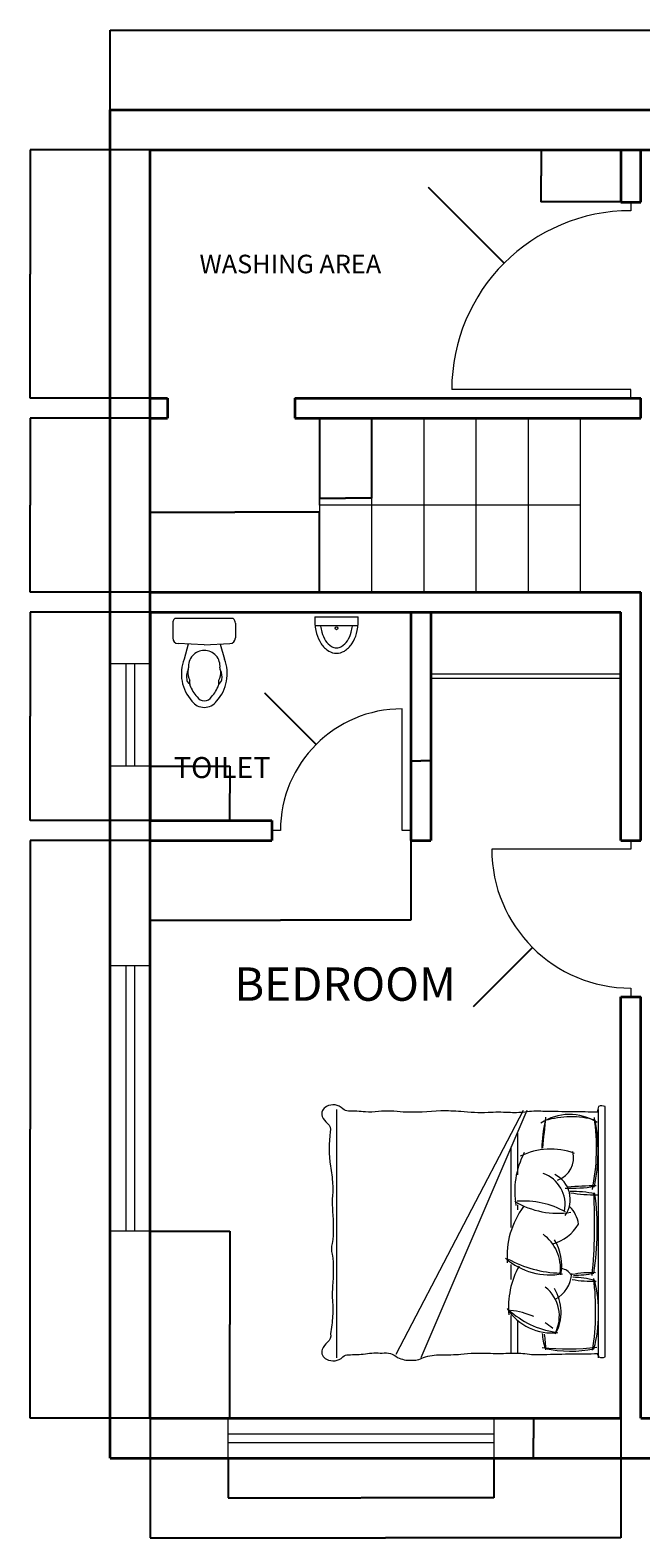
# Model space of a CAD drawing. Units: millimetres. Extents: x 2511 to 24632, y 2213 to 12972.
# Tile 1 of 5: x 2511 to 6023, y 2213 to 10891. Entities that reach past the tile are written whole.
import ezdxf

# ---------------------------------------------------------------- set-up
doc = ezdxf.new("R2010")
doc.units = ezdxf.units.MM
for name, color, linetype, lineweight in [('A-ANNO-DIMS', 2, 'Continuous', 18), ('A-AREA-IDEN', 7, 'Continuous', 20), ('A-FLOR-CASE', 7, 'Continuous', 18), ('A-FLOR-FIXT', 5, 'Continuous', 18), ('A-FLOR-STRS', 7, 'Continuous', 18), ('A-WALL', 7, 'Continuous', 35), ('doors', 50, 'Continuous', 18), ('windows', 70, 'Continuous', 18)]:
    doc.layers.add(name, color=color, linetype=linetype, lineweight=lineweight)
doc.layers.add('A-FURN', color=11, linetype='Continuous', lineweight=18, true_color=0xf27172)
doc.styles.get("Standard").update_dxf_attribs({"font": 'arial.ttf'})
doc.dimstyles.get("Standard").update_dxf_attribs({"dimtxt": 0.18, "dimasz": 0.18, "dimexe": 0.18, "dimexo": 0.0625, "dimgap": 0.09, "dimtad": 0, "dimtih": 1, "dimtoh": 1, "dimdec": 4, "dimzin": 0, "dimdsep": 46, "dimtxsty": 'Standard', "dimcen": 0.09, "dimadec": 0, "dimazin": 0, "dimtfac": 1, "dimtdec": 4, "dimtofl": 0, "dimtmove": 0, "dimatfit": 3, "dimfxl": 1, "dimtolj": 1, "dimtzin": 0, "dimarcsym": 0})

# ---------------------------------------------------------------- blocks, each defined once
blk = doc.blocks.new('WINDOW-1528-PLAN')
for p, q in [((0, 140), (1528, 140)), ((0, 90), (1528, 90))]:
    blk.add_line(p, q)
blk.add_lwpolyline([(0, 230), (1528, 230), (1528, 0), (0, 0)], close=True)
blk = doc.blocks.new('WINDOW-592-PLAN')
for p, q in [((0, 140), (591.5, 140)), ((0, 90), (591.5, 90))]:
    blk.add_line(p, q)
blk.add_lwpolyline([(0, 230), (591.5, 230), (591.5, 0), (0, 0)], close=True)
blk = doc.blocks.new('*D19')
at = {"layer": 'A-ANNO-DIMS', "color": 0, "lineweight": -2, "transparency": 16777216}
for p, q in [((3649.2, 2671.8), (3649.2, 2442.5)), ((5177.2, 2671.8), (5177.2, 2442.5)), ((3649.4, 2442.7), (4412, 2442.7)), ((5177, 2442.7), (4414.5, 2442.7))]:
    blk.add_line(p, q, dxfattribs=at)
at = {"layer": 'A-ANNO-DIMS', "color": 0, "transparency": 16777216}
for points in [[(3649.4, 2442.7), (3649.4, 2442.6), (3649.2, 2442.7)], [(5177, 2442.7), (5177, 2442.6), (5177.2, 2442.7)]]:
    blk.add_solid(points, dxfattribs=at)
at = {"layer": 'Defpoints', "color": 0, "transparency": 16777216}
for p in [(3649.2, 2671.9), (5177.2, 2671.9), (5177.2, 2442.7)]:
    blk.add_point(p, dxfattribs=at)
at = {"layer": 'A-ANNO-DIMS', "color": 0, "transparency": 16777216, "insert": (4413.2, 2442.7), "char_height": 0.18, "attachment_point": 5}
blk.add_mtext('\\A1;WINDOW 1528 TYP.', dxfattribs=at)
blk = doc.blocks.new('*D20')
at = {"layer": 'A-ANNO-DIMS', "color": 0, "lineweight": -2, "transparency": 16777216}
for p, q in [((5177.3, 2901.9), (5406.6, 2901.9)), ((5406.4, 2901.7), (5406.4, 2787)), ((5406.4, 2672), (5406.4, 2786.7)), ((5177.3, 2671.9), (5406.6, 2671.9))]:
    blk.add_line(p, q, dxfattribs=at)
at = {"layer": 'A-ANNO-DIMS', "color": 0, "transparency": 16777216}
for points in [[(5406.4, 2901.7), (5406.4, 2901.7), (5406.4, 2901.9)], [(5406.4, 2672), (5406.4, 2672), (5406.4, 2671.9)]]:
    blk.add_solid(points, dxfattribs=at)
at = {"layer": 'Defpoints', "color": 0, "transparency": 16777216}
for p in [(5177.2, 2901.9), (5406.4, 2901.9), (5177.2, 2671.9)]:
    blk.add_point(p, dxfattribs=at)
at = {"layer": 'A-ANNO-DIMS', "color": 0, "transparency": 16777216, "insert": (5406.4, 2786.9), "char_height": 0.18, "attachment_point": 5}
blk.add_mtext('\\A1;230 TYP.', dxfattribs=at)
blk = doc.blocks.new('*D35')
at = {"layer": 'A-ANNO-DIMS', "color": 0, "lineweight": -2, "transparency": 16777216}
for p, q in [((2970.2, 10431.9), (2970.2, 10891)), ((2970.4, 10890.9), (7557.9, 10890.9)), ((12146, 10890.9), (7558.6, 10890.9)), ((12146.2, 7356.9), (12146.2, 10891))]:
    blk.add_line(p, q, dxfattribs=at)
at = {"layer": 'A-ANNO-DIMS', "color": 0, "transparency": 16777216}
for points in [[(2970.4, 10890.9), (2970.4, 10890.8), (2970.2, 10890.9)], [(12146, 10890.9), (12146, 10890.8), (12146.2, 10890.9)]]:
    blk.add_solid(points, dxfattribs=at)
at = {"layer": 'Defpoints', "color": 0, "transparency": 16777216}
for p in [(12146.2, 10890.9), (2970.2, 10431.9), (12146.2, 7356.9)]:
    blk.add_point(p, dxfattribs=at)
at = {"layer": 'A-ANNO-DIMS', "color": 0, "transparency": 16777216, "insert": (7558.2, 10890.9), "char_height": 0.18, "attachment_point": 5}
blk.add_mtext('\\A1;9176', dxfattribs=at)
blk = doc.blocks.new('*D37')
at = {"layer": 'A-ANNO-DIMS', "color": 0, "lineweight": -2, "transparency": 16777216}
for p, q in [((3200.2, 2901.8), (3200.2, 2212.7)), ((5908.2, 2901.8), (5908.2, 2212.7)), ((3200.4, 2212.9), (4553.9, 2212.9)), ((5908, 2212.9), (4554.6, 2212.9))]:
    blk.add_line(p, q, dxfattribs=at)
at = {"layer": 'A-ANNO-DIMS', "color": 0, "transparency": 16777216}
for points in [[(3200.4, 2212.9), (3200.4, 2212.8), (3200.2, 2212.9)], [(5908, 2212.9), (5908, 2212.8), (5908.2, 2212.9)]]:
    blk.add_solid(points, dxfattribs=at)
at = {"layer": 'Defpoints', "color": 0, "transparency": 16777216}
for p in [(3200.2, 2901.9), (5908.2, 2901.9), (5908.2, 2212.9)]:
    blk.add_point(p, dxfattribs=at)
at = {"layer": 'A-ANNO-DIMS', "color": 0, "transparency": 16777216, "insert": (4554.2, 2212.9), "char_height": 0.18, "attachment_point": 5}
blk.add_mtext('\\A1;2708', dxfattribs=at)
blk = doc.blocks.new('*D40')
at = {"layer": 'A-ANNO-DIMS', "color": 0, "lineweight": -2, "transparency": 16777216}
for p, q in [((3200.2, 6226.9), (2511, 6226.9)), ((2511.2, 6226.7), (2511.2, 4564.5)), ((2511.2, 2902), (2511.2, 4564.2)), ((3200.2, 2901.9), (2511, 2901.9))]:
    blk.add_line(p, q, dxfattribs=at)
at = {"layer": 'A-ANNO-DIMS', "color": 0, "transparency": 16777216}
for points in [[(2511.2, 6226.7), (2511.2, 6226.7), (2511.2, 6226.9)], [(2511.2, 2902), (2511.2, 2902), (2511.2, 2901.9)]]:
    blk.add_solid(points, dxfattribs=at)
at = {"layer": 'Defpoints', "color": 0, "transparency": 16777216}
for p in [(2511.2, 6226.9), (3200.2, 6226.9), (3200.2, 2901.9)]:
    blk.add_point(p, dxfattribs=at)
at = {"layer": 'A-ANNO-DIMS', "color": 0, "transparency": 16777216, "insert": (2511.2, 4564.4), "char_height": 0.18, "attachment_point": 5}
blk.add_mtext('\\A1;3325', dxfattribs=at)
blk = doc.blocks.new('*D41')
at = {"layer": 'A-ANNO-DIMS', "color": 0, "lineweight": -2, "transparency": 16777216}
for p, q in [((3200.2, 7541.9), (2511, 7541.9)), ((2511.2, 7541.7), (2511.2, 6942)), ((2511.2, 6342), (2511.2, 6941.7)), ((3200.2, 6341.9), (2511, 6341.9))]:
    blk.add_line(p, q, dxfattribs=at)
at = {"layer": 'A-ANNO-DIMS', "color": 0, "transparency": 16777216}
for points in [[(2511.2, 7541.7), (2511.2, 7541.7), (2511.2, 7541.9)], [(2511.2, 6342), (2511.2, 6342), (2511.2, 6341.9)]]:
    blk.add_solid(points, dxfattribs=at)
at = {"layer": 'Defpoints', "color": 0, "transparency": 16777216}
for p in [(2511.2, 7541.9), (3200.2, 7541.9), (3200.2, 6341.9)]:
    blk.add_point(p, dxfattribs=at)
at = {"layer": 'A-ANNO-DIMS', "color": 0, "transparency": 16777216, "insert": (2511.2, 6941.9), "char_height": 0.18, "attachment_point": 5}
blk.add_mtext('\\A1;1200', dxfattribs=at)
blk = doc.blocks.new('*D42')
at = {"layer": 'A-ANNO-DIMS', "color": 0, "lineweight": -2, "transparency": 16777216}
for p, q in [((3200.2, 8656.9), (2511, 8656.9)), ((2511.2, 8656.7), (2511.2, 8157)), ((2511.2, 7657), (2511.2, 8156.7)), ((3200.2, 7656.9), (2511, 7656.9))]:
    blk.add_line(p, q, dxfattribs=at)
at = {"layer": 'A-ANNO-DIMS', "color": 0, "transparency": 16777216}
for points in [[(2511.2, 8656.7), (2511.2, 8656.7), (2511.2, 8656.9)], [(2511.2, 7657), (2511.2, 7657), (2511.2, 7656.9)]]:
    blk.add_solid(points, dxfattribs=at)
at = {"layer": 'Defpoints', "color": 0, "transparency": 16777216}
for p in [(2511.2, 8656.9), (3200.2, 8656.9), (3200.2, 7656.9)]:
    blk.add_point(p, dxfattribs=at)
at = {"layer": 'A-ANNO-DIMS', "color": 0, "transparency": 16777216, "insert": (2511.2, 8156.9), "char_height": 0.18, "attachment_point": 5}
blk.add_mtext('\\A1;1000', dxfattribs=at)
blk = doc.blocks.new('*D43')
at = {"layer": 'A-ANNO-DIMS', "color": 0, "lineweight": -2, "transparency": 16777216}
for p, q in [((3200.2, 10201.9), (2511, 10201.9)), ((2511.2, 10201.7), (2511.2, 9487)), ((2511.2, 8772), (2511.2, 9486.7)), ((3200.2, 8771.9), (2511, 8771.9))]:
    blk.add_line(p, q, dxfattribs=at)
at = {"layer": 'A-ANNO-DIMS', "color": 0, "transparency": 16777216}
for points in [[(2511.2, 10201.7), (2511.2, 10201.7), (2511.2, 10201.9)], [(2511.2, 8772), (2511.2, 8772), (2511.2, 8771.9)]]:
    blk.add_solid(points, dxfattribs=at)
at = {"layer": 'Defpoints', "color": 0, "transparency": 16777216}
for p in [(2511.2, 10201.9), (3200.2, 10201.9), (3200.2, 8771.9)]:
    blk.add_point(p, dxfattribs=at)
at = {"layer": 'A-ANNO-DIMS', "color": 0, "transparency": 16777216, "insert": (2511.2, 9486.9), "char_height": 0.18, "attachment_point": 5}
blk.add_mtext('\\A1;1430', dxfattribs=at)
blk = doc.blocks.new('*D44')
at = {"layer": 'A-ANNO-DIMS', "color": 0, "lineweight": -2, "transparency": 16777216}
for p, q in [((3200.3, 3978.2), (3659.4, 3978.2)), ((3659.2, 3978), (3659.2, 3440.2)), ((3659.2, 2902), (3659.2, 3439.9)), ((3200.3, 2901.9), (3659.4, 2901.9))]:
    blk.add_line(p, q, dxfattribs=at)
at = {"layer": 'A-ANNO-DIMS', "color": 0, "transparency": 16777216}
for points in [[(3659.2, 3978), (3659.2, 3978), (3659.2, 3978.2)], [(3659.2, 2902), (3659.2, 2902), (3659.2, 2901.9)]]:
    blk.add_solid(points, dxfattribs=at)
at = {"layer": 'Defpoints', "color": 0, "transparency": 16777216}
for p in [(3200.2, 3978.2), (3200.2, 2901.9), (3659.2, 2901.9)]:
    blk.add_point(p, dxfattribs=at)
at = {"layer": 'A-ANNO-DIMS', "color": 0, "transparency": 16777216, "insert": (3659.2, 3440), "char_height": 0.18, "attachment_point": 5}
blk.add_mtext('\\A1;1076.3', dxfattribs=at)
blk = doc.blocks.new('*D45')
at = {"layer": 'A-ANNO-DIMS', "color": 0, "lineweight": -2, "transparency": 16777216}
for p, q in [((3200.3, 6654.5), (3659.4, 6654.5)), ((3659.2, 6654.4), (3659.2, 6498.4)), ((3659.2, 6342), (3659.2, 6498)), ((3200.3, 6341.9), (3659.4, 6341.9))]:
    blk.add_line(p, q, dxfattribs=at)
at = {"layer": 'A-ANNO-DIMS', "color": 0, "transparency": 16777216}
for points in [[(3659.2, 6654.4), (3659.2, 6654.4), (3659.2, 6654.5)], [(3659.2, 6342), (3659.2, 6342), (3659.2, 6341.9)]]:
    blk.add_solid(points, dxfattribs=at)
at = {"layer": 'Defpoints', "color": 0, "transparency": 16777216}
for p in [(3200.2, 6654.5), (3200.2, 6341.9), (3659.2, 6341.9)]:
    blk.add_point(p, dxfattribs=at)
at = {"layer": 'A-ANNO-DIMS', "color": 0, "transparency": 16777216, "insert": (3659.2, 6498.2), "char_height": 0.18, "attachment_point": 5}
blk.add_mtext('\\A1;312.7', dxfattribs=at)
blk = doc.blocks.new('*D46')
at = {"layer": 'A-ANNO-DIMS', "color": 0, "lineweight": -2, "transparency": 16777216}
for p, q in [((3200.2, 6226.8), (3200.2, 5767.7)), ((4700.2, 6226.8), (4700.2, 5767.7)), ((3200.4, 5767.9), (3949.9, 5767.9)), ((4700, 5767.9), (3950.6, 5767.9))]:
    blk.add_line(p, q, dxfattribs=at)
at = {"layer": 'A-ANNO-DIMS', "color": 0, "transparency": 16777216}
for points in [[(3200.4, 5767.9), (3200.4, 5767.8), (3200.2, 5767.9)], [(4700, 5767.9), (4700, 5767.8), (4700.2, 5767.9)]]:
    blk.add_solid(points, dxfattribs=at)
at = {"layer": 'Defpoints', "color": 0, "transparency": 16777216}
for p in [(3200.2, 6226.9), (4700.2, 6226.9), (3200.2, 5767.9)]:
    blk.add_point(p, dxfattribs=at)
at = {"layer": 'A-ANNO-DIMS', "color": 0, "transparency": 16777216, "insert": (3950.2, 5767.9), "char_height": 0.18, "attachment_point": 5}
blk.add_mtext('\\A1;1500', dxfattribs=at)
blk = doc.blocks.new('*D47')
at = {"layer": 'A-ANNO-DIMS', "color": 0, "lineweight": -2, "transparency": 16777216}
for p, q in [((4700.2, 6226.9), (4700.2, 6686)), ((4700.4, 6685.9), (4757.4, 6685.9)), ((4815, 6685.9), (4758, 6685.9)), ((4815.2, 6226.9), (4815.2, 6686))]:
    blk.add_line(p, q, dxfattribs=at)
at = {"layer": 'A-ANNO-DIMS', "color": 0, "transparency": 16777216}
for points in [[(4700.4, 6685.9), (4700.4, 6685.8), (4700.2, 6685.9)], [(4815, 6685.9), (4815, 6685.8), (4815.2, 6685.9)]]:
    blk.add_solid(points, dxfattribs=at)
at = {"layer": 'Defpoints', "color": 0, "transparency": 16777216}
for p in [(4815.2, 6685.9), (4700.2, 6226.9), (4815.2, 6226.9)]:
    blk.add_point(p, dxfattribs=at)
at = {"layer": 'A-ANNO-DIMS', "color": 0, "transparency": 16777216, "insert": (4757.7, 6685.9), "char_height": 0.18, "attachment_point": 5}
blk.add_mtext('\\A1;115', dxfattribs=at)
blk = doc.blocks.new('*D48')
at = {"layer": 'A-ANNO-DIMS', "color": 0, "lineweight": -2, "transparency": 16777216}
for p, q in [((4174.9, 8656.8), (4174.9, 8197.7)), ((4474.9, 8656.8), (4474.9, 8197.7)), ((4175.1, 8197.9), (4324.7, 8197.9)), ((4474.8, 8197.9), (4325.2, 8197.9))]:
    blk.add_line(p, q, dxfattribs=at)
at = {"layer": 'A-ANNO-DIMS', "color": 0, "transparency": 16777216}
for points in [[(4175.1, 8197.9), (4175.1, 8197.8), (4174.9, 8197.9)], [(4474.8, 8197.9), (4474.8, 8197.8), (4474.9, 8197.9)]]:
    blk.add_solid(points, dxfattribs=at)
at = {"layer": 'Defpoints', "color": 0, "transparency": 16777216}
for p in [(4174.9, 8656.9), (4474.9, 8656.9), (4174.9, 8197.9)]:
    blk.add_point(p, dxfattribs=at)
at = {"layer": 'A-ANNO-DIMS', "color": 0, "transparency": 16777216, "insert": (4324.9, 8197.9), "char_height": 0.18, "attachment_point": 5}
blk.add_mtext('\\A1;300', dxfattribs=at)
blk = doc.blocks.new('*D49')
at = {"layer": 'A-ANNO-DIMS', "color": 0, "lineweight": -2, "transparency": 16777216}
for p, q in [((3200.2, 7656.9), (3200.2, 8116)), ((3200.4, 8115.9), (3687.2, 8115.9)), ((4174.8, 8115.9), (3688, 8115.9)), ((4174.9, 7656.9), (4174.9, 8116))]:
    blk.add_line(p, q, dxfattribs=at)
at = {"layer": 'A-ANNO-DIMS', "color": 0, "transparency": 16777216}
for points in [[(3200.4, 8115.9), (3200.4, 8115.8), (3200.2, 8115.9)], [(4174.8, 8115.9), (4174.8, 8115.8), (4174.9, 8115.9)]]:
    blk.add_solid(points, dxfattribs=at)
at = {"layer": 'Defpoints', "color": 0, "transparency": 16777216}
for p in [(4174.9, 8115.9), (3200.2, 7656.9), (4174.9, 7656.9)]:
    blk.add_point(p, dxfattribs=at)
at = {"layer": 'A-ANNO-DIMS', "color": 0, "transparency": 16777216, "insert": (3687.6, 8115.9), "char_height": 0.18, "attachment_point": 5}
blk.add_mtext('\\A1;974.7', dxfattribs=at)
blk = doc.blocks.new('*D63')
at = {"layer": 'A-ANNO-DIMS', "color": 0, "lineweight": -2, "transparency": 16777216}
for p, q in [((5908.2, 10201.9), (5449, 10201.9)), ((5449.2, 10201.7), (5449.2, 10052)), ((5449.2, 9902), (5449.2, 10051.7)), ((5908.2, 9901.9), (5449, 9901.9))]:
    blk.add_line(p, q, dxfattribs=at)
at = {"layer": 'A-ANNO-DIMS', "color": 0, "transparency": 16777216}
for points in [[(5449.2, 10201.7), (5449.2, 10201.7), (5449.2, 10201.9)], [(5449.2, 9902), (5449.2, 9902), (5449.2, 9901.9)]]:
    blk.add_solid(points, dxfattribs=at)
at = {"layer": 'Defpoints', "color": 0, "transparency": 16777216}
for p in [(5449.2, 10201.9), (5908.2, 10201.9), (5908.2, 9901.9)]:
    blk.add_point(p, dxfattribs=at)
at = {"layer": 'A-ANNO-DIMS', "color": 0, "transparency": 16777216, "insert": (5449.2, 10051.9), "char_height": 0.18, "attachment_point": 5}
blk.add_mtext('\\A1;300', dxfattribs=at)
blk = doc.blocks.new('*D97')
at = {"layer": 'A-ANNO-DIMS', "color": 0, "lineweight": -2, "transparency": 16777216}
for p, q in [((4800.2, 9987.2), (4800.4, 9987.2)), ((4800.4, 9987.2), (5237.3, 9550.3)), ((5965.6, 8821.9), (5965.8, 8821.9)), ((5965.7, 8821.8), (5965.7, 8822))]:
    blk.add_line(p, q, dxfattribs=at)
at = {"layer": 'A-ANNO-DIMS', "color": 0, "transparency": 16777216}
blk.add_solid([(5237.3, 9550.3), (5237.2, 9550.3), (5237.4, 9550.2)], dxfattribs=at)
at = {"layer": 'Defpoints', "color": 0, "transparency": 16777216}
for p in [(5237.4, 9550.2), (5965.7, 8821.9)]:
    blk.add_point(p, dxfattribs=at)
at = {"layer": 'A-ANNO-DIMS', "color": 0, "transparency": 16777216, "insert": (4799.8, 9987.2), "char_height": 0.18, "attachment_point": 5}
blk.add_mtext('\\A1;R1030', dxfattribs=at)
blk = doc.blocks.new('*D98')
at = {"layer": 'A-ANNO-DIMS', "color": 0, "lineweight": -2, "transparency": 16777216}
for p, q in [((5965.6, 6176.9), (5965.8, 6176.9)), ((5965.7, 6176.8), (5965.7, 6177)), ((5060.6, 5271.8), (5399.9, 5611.1)), ((5060.4, 5271.8), (5060.6, 5271.8))]:
    blk.add_line(p, q, dxfattribs=at)
at = {"layer": 'A-ANNO-DIMS', "color": 0, "transparency": 16777216}
blk.add_solid([(5399.9, 5611.1), (5399.9, 5611), (5400, 5611.2)], dxfattribs=at)
at = {"layer": 'Defpoints', "color": 0, "transparency": 16777216}
for p in [(5965.7, 6176.9), (5400, 5611.2)]:
    blk.add_point(p, dxfattribs=at)
at = {"layer": 'A-ANNO-DIMS', "color": 0, "transparency": 16777216, "insert": (5060.1, 5271.8), "char_height": 0.18, "attachment_point": 5}
blk.add_mtext('\\A1;R800', dxfattribs=at)
blk = doc.blocks.new('*D100')
at = {"layer": 'A-ANNO-DIMS', "color": 0, "lineweight": -2, "transparency": 16777216}
for p, q in [((3858.1, 7076.3), (3858.3, 7076.3)), ((3858.3, 7076.3), (4155.1, 6779.5)), ((4650.1, 6284.4), (4650.3, 6284.4)), ((4650.2, 6284.3), (4650.2, 6284.5))]:
    blk.add_line(p, q, dxfattribs=at)
at = {"layer": 'A-ANNO-DIMS', "color": 0, "transparency": 16777216}
blk.add_solid([(4155.1, 6779.5), (4155.1, 6779.4), (4155.2, 6779.3)], dxfattribs=at)
at = {"layer": 'Defpoints', "color": 0, "transparency": 16777216}
for p in [(4155.2, 6779.3), (4650.2, 6284.4)]:
    blk.add_point(p, dxfattribs=at)
at = {"layer": 'A-ANNO-DIMS', "color": 0, "transparency": 16777216, "insert": (3857.7, 7076.3), "char_height": 0.18, "attachment_point": 5}
blk.add_mtext('\\A1;R700', dxfattribs=at)

msp = doc.modelspace()

# ---------------------------------------------------------------- linework, layer by layer
at = {"layer": 'A-FLOR-CASE'}
for p, q in [((4815.215, 7186.544), (5908.215, 7186.544)), ((4815.215, 7161.544), (5908.215, 7161.544))]:
    msp.add_line(p, q, dxfattribs=at)
at = {"layer": 'A-FLOR-FIXT', "ltscale": 20}
for p, q in [((3330.928, 7478.078), (3330.928, 7392.343)), ((3677.016, 7504.669), (3344.929, 7504.669)), ((3691.017, 7478.078), (3691.017, 7392.343)), ((3510.973, 7353.464), (3361.678, 7360.179)), ((3420.522, 7357.532), (3396.973, 7271.135)), ((3510.973, 7353.464), (3660.267, 7360.179)), ((3604.275, 7357.66), (3627.859, 7271.135)), ((3425.384, 7130.445), (3415.315, 7142.445)), ((3428.864, 7127.47), (3428.864, 7149.787)), ((3595.968, 7127.47), (3595.968, 7149.787)), ((3599.448, 7130.445), (3609.517, 7142.445))]:
    msp.add_line(p, q, dxfattribs=at)
at = {"layer": 'A-FLOR-FIXT'}
for p, q in [((4148.635, 7514.291), (4397.234, 7514.291)), ((4152.312, 7464.195), (4393.557, 7464.195))]:
    msp.add_line(p, q, dxfattribs=at)
for points in [[(4148.635, 7514.291, 0.01969394), (4147.765, 7492.208, 0.06745904), (4157.89, 7417.504, 0.07981249), (4184.426, 7359.446, 0.10711811), (4227.956, 7317.289, 0.13988915), (4272.934, 7304.454, 0.13988915)], [(4272.934, 7304.454, 0.13988915), (4317.912, 7317.289, 0.10711811), (4361.442, 7359.446, 0.07981249), (4387.979, 7417.504, 0.06745904), (4398.104, 7492.208, 0.01969394), (4397.234, 7514.291, 0.02043933)], [(4181.01, 7461.066, 0.03606883), (4188.053, 7425.833, 0.07981249), (4210.463, 7376.804, 0.10711811), (4244.471, 7343.869, 0.13988915), (4272.934, 7335.746, 0.13988915)], [(4272.934, 7335.746, 0.13988915), (4301.398, 7343.869, 0.10711811), (4335.406, 7376.804, 0.07981249), (4357.815, 7425.833, 0.03606883), (4364.859, 7461.066, 0.02217222)]]:
    msp.add_lwpolyline(points, format="xyb", dxfattribs=at)
msp.add_circle((4272.934, 7448.375), 8.507, dxfattribs=at)
at = {"layer": 'A-FLOR-FIXT', "ltscale": 20}
for centre, radius, start, end in [((3365.867, 7478.078), 34.939, 133.4731092, 180), ((3344.929, 7500.162), 4.507, 90, 133.4731092), ((3677.016, 7500.162), 4.507, 46.5268908, 90), ((3656.078, 7478.078), 34.939, 0, 46.5268908), ((3363.125, 7392.343), 32.197, 180, 267.4244631), ((3658.82, 7392.343), 32.197, 272.5755369, 0), ((3512.416, 7230.196), 90.633, 90, 186.6477367), ((3512.416, 7230.196), 90.633, 353.3522633, 90), ((3610.973, 7185.574), 230.47, 158.2075947, 222.5865487), ((3495.89, 7167.095), 86.201, 151.425845, 190.6031704), ((3403.365, 7217.486), 19.156, 331.425845, 6.6477367), ((3413.859, 7185.574), 230.47, 317.4134513, 21.7924053), ((3621.467, 7217.486), 19.156, 173.3522633, 208.574155), ((3528.943, 7167.095), 86.201, 349.3968296, 28.574155), ((3429.989, 7154.758), 19.156, 190.6031704, 220), ((3531.724, 7200.457), 114.935, 179.5478357, 206.4979771), ((3410.71, 7118.132), 19.156, 18.6118763, 40), ((3448.019, 7127.47), 19.156, 180, 199.6248963), ((3610.973, 7185.574), 192.159, 199.6248963, 223.3880194), ((3413.859, 7185.574), 192.159, 316.6119806, 340.3751037), ((3576.813, 7127.47), 19.156, 340.3751037, 0), ((3493.108, 7200.457), 114.935, 333.5020229, 0.4521643), ((3614.122, 7118.132), 19.156, 140, 161.3881237), ((3594.843, 7154.758), 19.156, 320, 349.3968296), ((3512.416, 7079.955), 87.14, 215.2885251, 270), ((3512.416, 7079.955), 48.828, 212.7026161, 270), ((3512.416, 7079.955), 48.828, 270, 327.2973839), ((3512.416, 7079.955), 87.14, 270, 324.7114749)]:
    msp.add_arc(centre, radius, start, end, dxfattribs=at)
at = {"layer": 'A-FLOR-STRS'}
for p, q in [((4174.942, 8156.864), (4174.942, 8656.864)), ((4174.942, 8656.864), (4174.942, 7656.864)), ((4474.942, 8656.864), (4474.942, 7656.864)), ((4774.942, 8656.864), (4774.942, 7656.864)), ((5074.942, 8656.864), (5074.942, 7656.864)), ((5374.942, 8656.864), (5374.942, 7656.864)), ((5674.942, 8656.864), (5674.942, 7656.864)), ((5674.942, 8156.864), (4174.942, 8156.864))]:
    msp.add_line(p, q, dxfattribs=at)
at = {"layer": 'A-FURN'}
for p, q in [((4273.444, 4678.817), (4273.444, 3247.992)), ((5345.679, 4671.712), (4614.401, 3267.571)), ((5368.531, 4671.712), (4758.044, 3247.992)), ((5777.254, 4678.817), (5777.254, 3247.992)), ((5313.56, 4541.541), (5313.56, 4303.027)), ((5274.919, 4463.675), (5274.919, 3999.391)), ((5313.56, 4128.609), (5313.56, 4100.459)), ((5274.919, 3785.735), (5274.919, 3699.74)), ((5274.919, 3492.926), (5274.919, 3276.185)), ((5313.56, 3463.149), (5313.56, 3276.318))]:
    msp.add_line(p, q, dxfattribs=at)
msp.add_lwpolyline([(5773.346, 3274.098, 0.09869851), (5781.605, 3254.627, 0.22252235), (5817.884, 3254.627), (5817.884, 4695.411, 0.17162122), (5780.166, 4696.243, 0.10249488), (5773.346, 4662.15, 0.01557073), (5634.111, 4664.028, 0.00267017), (5460.281, 4667.674, 0.05895767), (5356.051, 4662.604, -0.03845753), (5261.954, 4660.654, 0.02550828), (5144.632, 4660.654, -0.0394122), (4987.963, 4666.552, 0.0164979), (4873.846, 4670.818, -0.03577068), (4657.185, 4663.631, 0.04538792), (4513.719, 4667.685, -0.0805782), (4439.036, 4664.164, 0.0265044), (4341.24, 4669.282, -0.21113367), (4310.049, 4682.138, 0.32944645), (4215.103, 4695.055, 0.37589027), (4189.792, 4638.587, 0.12389154), (4221.298, 4598.015, -0.34253901), (4236.785, 4550.486, 0.07104041), (4238.678, 4352.482, -0.03644179), (4250.159, 4249.825, -0.04679119), (4248.667, 4167.055, 0.02362788), (4250.256, 4090.987, -0.05589674), (4248.394, 3906.836, 0.05352755), (4243.208, 3876.006, 0.05352755), (4248.394, 3845.175, -0.05589674), (4250.256, 3661.025, 0.02697324), (4248.667, 3594.395, -0.03694731), (4250.159, 3489.566, -0.03644179), (4238.678, 3386.909, -0.28125631), (4221.298, 3338.233, -0.52199546), (4221.298, 3338.233, 0.12389154), (4189.792, 3297.661, 0.37589027), (4215.103, 3241.193, 0.32944645), (4310.049, 3254.111, -0.21113367), (4341.24, 3266.966, 0.0265044), (4439.036, 3272.084, -0.06219016), (4535.843, 3275.655, -0.21823319), (4624.171, 3250.825, 0.12351304), (4700.169, 3234.608, 0.12988697), (4773.128, 3250.319, -0.09506344), (4873.846, 3265.43, 0.0164979), (4987.963, 3269.696, -0.0394122), (5144.632, 3275.594, 0.02550828), (5261.954, 3275.594, -0.03845753), (5356.051, 3273.644, 0.05895767), (5460.281, 3268.574, 0.00267017), (5634.111, 3272.22, 0.01557073)], format="xyb", close=True, dxfattribs=at)
for centre, radius, start, end in [((5612.879, 4354.272), 295.69, 57.5099621, 123.8335945), ((6404.497, 4418.051), 951.942, 168.1169154, 177.8849264), ((-2129.276, 5360.107), 7641.5, 353.2132218, 354.5476162), ((5621.346, 4132.938), 503.496, 73.9263495, 107.1408686), ((4560.481, 4456.811), 1208.201, 348.5485317, 8.3029026), ((4798.04, 4438.106), 979.146, 348.0142101, 10.5124793), ((5777.12, 4207.667), 479.253, 152.3858681, 189.8950776), ((5503.906, 4060.43), 390.033, 69.302573, 116.5026347), ((5500.067, 4401.854), 137.12, 288.9386924, 14.6725101), ((5398.568, 4132.224), 188.955, 348.0412562, 70.8342262), ((5458.948, 4161.667), 158.335, 324.167062, 63.8421297), ((5605.348, 5369.704), 1144.871, 269.1535781, 277.5532947), ((5770.251, 2022.742), 2215.701, 90.1062848, 94.3311669), ((5615.988, 3419.347), 787.622, 79.5301281, 89.9340478), ((5748.071, 4906.613), 719.223, 259.5889949, 272.0446713), ((2741.329, 4019.396), 3016.27, 354.365794, 3.396867), ((4176.802, 3987.603), 1595.698, 350.9339646, 7.4265878), ((5732.186, 3833.042), 478.701, 143.2201032, 184.4972467), ((5545.448, 4556.056), 475.262, 238.6541912, 279.1976874), ((5347.563, 3649.972), 501.613, 61.0455512, 94.1496924), ((5499.059, 3998.675), 166.504, 6.8992405, 46.0420784), ((5452.194, 4142.593), 245.7, 285.4017561, 329.7122045), ((5319.495, 3763.612), 241.725, 353.5606615, 54.285295), ((5293.523, 3782.692), 274.731, 348.4080606, 32.0077461), ((5501.428, 4118.666), 392.279, 229.1338862, 280.5298924), ((5580.82, 4412.217), 676.148, 241.6049526, 268.1748992), ((5746.627, 3541.897), 484.517, 150.9467315, 185.4670485), ((5445.666, 3745.271), 180.605, 298.1995589, 356.5060516), ((5562.281, 3693.19), 68.36, 30.1134148, 85.8974179), ((5740.291, 3178.116), 561.004, 87.826075, 101.4767373), ((5611.771, 4481.691), 758.705, 271.8336993, 280.694498), ((5343.086, 3489.507), 211.654, 331.8876328, 51.870713), ((5302.015, 3511.697), 262.423, 331.6403939, 31.3344793), ((5735.3, 4257.319), 567.333, 259.1666567, 273.1229689), ((5616.281, 3153.013), 559.709, 75.3433978, 88.3875666), ((4233.38, 3522.008), 1530.055, 351.3713579, 6.9170324), ((4986.99, 3506.023), 793.62, 345.0181287, 13.7391648), ((5509.733, 3694.15), 301.926, 212.3262293, 277.0000098), ((5606.252, 3896.848), 505.784, 227.3201338, 261.4624014), ((5225.963, 3072.502), 451.755, 66.2981822, 83.8538565), ((5873.832, 3428.941), 420.146, 185.4469786, 197.4198666), ((4928.493, 3287.839), 548.761, 0.6431821, 10.2706619), ((5225.963, 3072.502), 451.755, 49.9508295, 56.9510198), ((5605.319, 4755.244), 1455.067, 264.0935071, 276.4707411), ((5618.607, 3950.393), 663.418, 257.3175056, 281.7434533)]:
    msp.add_arc(centre, radius, start, end, dxfattribs=at)
at = {"layer": 'A-WALL'}
for p, q in [((2970.215, 2671.864), (2970.215, 10431.864)), ((2970.215, 10431.864), (11740.215, 10431.864)), ((3200.215, 10201.864), (6023.215, 10201.864)), ((3200.215, 8771.864), (3200.215, 10201.864)), ((5908.215, 10201.864), (5908.215, 9901.864)), ((6023.215, 10201.864), (10200.215, 10201.864)), ((6023.215, 9901.864), (6023.215, 10201.864)), ((5908.215, 9901.864), (6023.215, 9901.864)), ((3200.215, 2901.864), (3200.215, 8771.864)), ((3200.215, 8771.864), (3300.215, 8771.864)), ((3300.215, 8771.864), (3300.215, 8656.864)), ((4033.102, 8771.864), (4033.102, 8656.864)), ((4033.102, 8771.864), (6023.215, 8771.864)), ((6023.215, 8656.864), (6023.215, 8771.864)), ((3200.215, 8656.864), (3300.215, 8656.864)), ((4033.102, 8656.864), (6023.215, 8656.864)), ((3200.215, 7656.864), (6023.215, 7656.864)), ((6023.215, 6226.864), (6023.215, 7656.864)), ((3200.215, 7541.864), (5908.215, 7541.864)), ((3200.215, 7541.864), (3200.215, 6341.864)), ((4700.215, 7541.864), (4700.215, 6341.864)), ((4815.215, 7541.864), (4815.215, 6226.864)), ((5908.215, 6226.864), (5908.215, 7541.864)), ((3200.215, 6341.864), (3900.215, 6341.864)), ((3900.215, 6341.864), (3900.215, 6226.864)), ((4700.215, 6341.864), (4700.215, 6226.864)), ((3200.215, 6226.864), (3900.215, 6226.864)), ((4700.215, 6226.864), (4815.215, 6226.864)), ((5908.215, 6226.864), (6023.215, 6226.864)), ((5908.215, 2901.864), (5908.215, 5326.864)), ((5908.215, 5326.864), (6023.215, 5326.864)), ((6023.215, 2901.864), (6023.215, 5326.864)), ((3200.215, 2901.864), (5908.215, 2901.864)), ((6023.215, 2901.864), (8051.215, 2901.864)), ((2970.215, 2671.864), (8051.215, 2671.864))]:
    msp.add_line(p, q, dxfattribs=at)
at = {"layer": 'doors'}
for p, q in [((5965.715, 9901.864), (5965.715, 9851.864)), ((5965.715, 8821.864), (4935.715, 8821.864)), ((5965.715, 8771.864), (5965.715, 8821.864)), ((4650.215, 6284.364), (4650.215, 6984.364)), ((4700.215, 6341.864), (4700.215, 6226.864)), ((3950.215, 6284.364), (3900.215, 6284.364)), ((4700.215, 6284.364), (4650.215, 6284.364)), ((5965.715, 6176.864), (5165.715, 6176.864)), ((5908.215, 6226.864), (6023.215, 6226.864)), ((5965.715, 6226.864), (5965.715, 6176.864)), ((5965.715, 5376.864), (5965.715, 5326.864))]:
    msp.add_line(p, q, dxfattribs=at)
for centre, radius, start, end in [((5965.715, 8821.864), 1030, 90, 180), ((4650.215, 6284.364), 700, 90, 180), ((5965.715, 6176.864), 800, 180, 270)]:
    msp.add_arc(centre, radius, start, end, dxfattribs=at)

# ---------------------------------------------------------------- block references
at = {"layer": 'windows', "rotation": 270}
for name, p in [('WINDOW-592-PLAN', (2970.215, 7246.089)), ('WINDOW-1528-PLAN', (2970.215, 5506.189))]:
    msp.add_blockref(name, p, dxfattribs=at)
at = {"layer": 'windows'}
msp.add_blockref('WINDOW-1528-PLAN', (3649.22, 2671.864), dxfattribs=at)

# ---------------------------------------------------------------- texts
at = {"layer": 'A-AREA-IDEN', "attachment_point": 1}
for s, width, gutter_width, insert, char_height in [('{\\fArial|b1|i0|c0|p34;WASHING AREA}', 1252.07649, 533.548, (3484.848, 9598.337), 106.70956), ('{\\fArial|b1|i0|c0|p34;TOILET}', 618.99213, 605.738, (3337.435, 6707.043), 121.14764), ('{\\fArial|b1|i0|c0|p34;BEDROOM}', 192.13251, 96.066, (3684.829, 5496.151), 192.13251)]:
    msp.add_mtext_dynamic_manual_height_columns(s, width=width, gutter_width=gutter_width, heights=[0], dxfattribs=dict(at, insert=insert, char_height=char_height))

# ---------------------------------------------------------------- dimensions: what is measured, and where the dimension line sits
at = {"layer": 'A-ANNO-DIMS'}
for base, p1, p2, picture, middle in [((12146.215, 10890.864), (2970.215, 10431.864), (12146.215, 7356.864), '*D35', (7558.215, 10890.864)), ((4815.215, 6685.864), (4700.215, 6226.864), (4815.215, 6226.864), '*D47', (4757.715, 6685.864)), ((5908.215, 2212.864), (3200.215, 2901.864), (5908.215, 2901.864), '*D37', (4554.215, 2212.864))]:
    dim = msp.add_linear_dim(base=base, p1=p1, p2=p2, dimstyle='Standard', override={"dimdec": 0, "dimlfac": 1, "dimrnd": 0, "dimzin": 0, "dimdsep": 46, "dimlunit": 2}, dxfattribs=at)
    dim.commit()
    dim.dimension.update_dxf_attribs({"geometry": picture, "text_midpoint": middle})
for base, p1, p2, angle, override, picture, middle in [((2511.215, 10201.864), (3200.215, 8771.864), (3200.215, 10201.864), 90, {"dimdec": 0, "dimlfac": 1, "dimrnd": 0, "dimzin": 0, "dimdsep": 46, "dimlunit": 2}, '*D43', (2511.215, 9486.864)), ((5449.215, 10201.864), (5908.215, 9901.864), (5908.215, 10201.864), 90, {"dimdec": 0, "dimlfac": 1, "dimrnd": 0, "dimzin": 0, "dimdsep": 46, "dimlunit": 2}, '*D63', (5449.215, 10051.864)), ((2511.215, 8656.864), (3200.215, 7656.864), (3200.215, 8656.864), 90, {"dimdec": 0, "dimlfac": 1, "dimrnd": 0, "dimzin": 0, "dimdsep": 46, "dimlunit": 2}, '*D42', (2511.215, 8156.864)), ((4174.942, 8197.864), (4474.942, 8656.864), (4174.942, 8656.864), 180, {"dimdec": 0, "dimlfac": 1, "dimrnd": 0, "dimzin": 0, "dimdsep": 46, "dimlunit": 2}, '*D48', (4324.942, 8197.864)), ((4174.942, 8115.864), (3200.215, 7656.864), (4174.942, 7656.864), 0, {"dimdec": 1, "dimlfac": 1, "dimrnd": 0, "dimzin": 0, "dimdsep": 46, "dimlunit": 2}, '*D49', (3687.578, 8115.864)), ((2511.215, 7541.864), (3200.215, 6341.864), (3200.215, 7541.864), 90, {"dimdec": 0, "dimlfac": 1, "dimrnd": 0, "dimzin": 0, "dimdsep": 46, "dimlunit": 2}, '*D41', (2511.215, 6941.864)), ((3659.215, 6341.864), (3200.215, 6654.541), (3200.215, 6341.864), 270, {"dimdec": 1, "dimlfac": 1, "dimrnd": 0, "dimzin": 0, "dimdsep": 46, "dimlunit": 2}, '*D45', (3659.215, 6498.202)), ((2511.215, 6226.864), (3200.215, 2901.864), (3200.215, 6226.864), 90, {"dimdec": 0, "dimlfac": 1, "dimrnd": 0, "dimzin": 0, "dimdsep": 46, "dimlunit": 2}, '*D40', (2511.215, 4564.364)), ((3200.215, 5767.864), (4700.215, 6226.864), (3200.215, 6226.864), 180, {"dimdec": 0, "dimlfac": 1, "dimrnd": 0, "dimzin": 0, "dimdsep": 46, "dimlunit": 2}, '*D46', (3950.215, 5767.864)), ((3659.215, 2901.864), (3200.215, 3978.201), (3200.215, 2901.864), 270, {"dimdec": 1, "dimlfac": 1, "dimrnd": 0, "dimzin": 0, "dimdsep": 46, "dimlunit": 2}, '*D44', (3659.215, 3440.032))]:
    dim = msp.add_linear_dim(base=base, p1=p1, p2=p2, angle=angle, dimstyle='Standard', override=override, dxfattribs=at)
    dim.commit()
    dim.dimension.update_dxf_attribs({"geometry": picture, "text_midpoint": middle})
for center, mpoint, picture, middle in [((5965.715, 8821.864), (5237.395, 9550.184), '*D97', (4799.779, 9987.176)), ((4650.215, 6284.364), (4155.24, 6779.339), '*D100', (3857.701, 7076.324)), ((5965.715, 6176.864), (5400.029, 5611.178), '*D98', (5060.063, 5271.767))]:
    dim = msp.add_radius_dim(center=center, mpoint=mpoint, dimstyle='Standard', override={"dimdec": 0, "dimlfac": 1, "dimrnd": 0, "dimzin": 0, "dimdsep": 46, "dimlunit": 2}, dxfattribs=at)
    dim.commit()
    dim.dimension.update_dxf_attribs({"geometry": picture, "text_midpoint": middle, "dimtype": 164})
dim = msp.add_linear_dim(base=(5406.406, 2901.864), p1=(5177.208, 2671.864), p2=(5177.208, 2901.864), angle=90, text='<> TYP.', dimstyle='Standard', override={"dimdec": 0, "dimlfac": 1, "dimrnd": 0, "dimzin": 0, "dimdsep": 46, "dimlunit": 2}, dxfattribs=at)
dim.commit()
dim.dimension.update_dxf_attribs({"geometry": '*D20', "text_midpoint": (5406.406, 2786.864)})
dim = msp.add_linear_dim(base=(5177.208, 2442.666), p1=(3649.22, 2671.864), p2=(5177.208, 2671.864), text='WINDOW <> TYP.', dimstyle='Standard', override={"dimdec": 0, "dimlfac": 1, "dimrnd": 0, "dimzin": 0, "dimdsep": 46, "dimlunit": 2}, dxfattribs=at)
dim.commit()
dim.dimension.update_dxf_attribs({"geometry": '*D19', "text_midpoint": (4413.214, 2442.666)})

doc.saveas('drawing.dxf')
